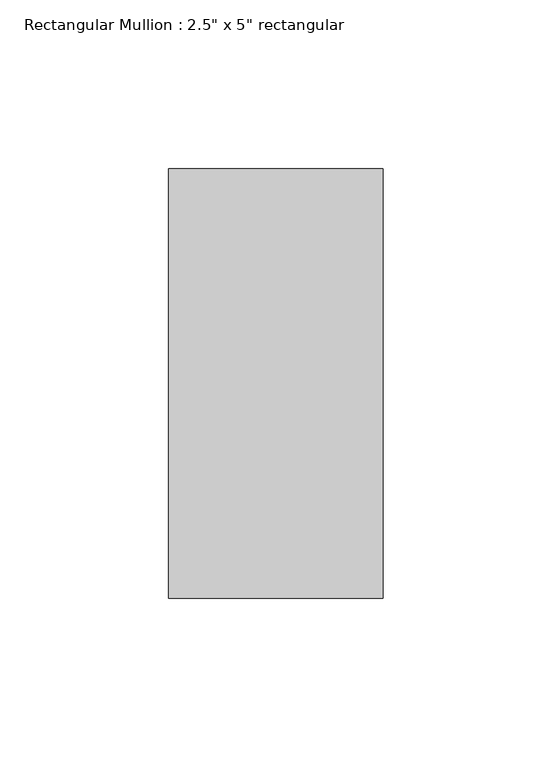
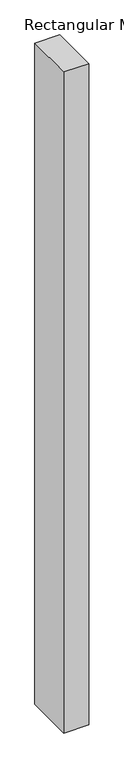
"""IFC4 building model written with IfcOpenShell, lengths in millimetres: member geometry."""

from ifc_helpers import new_model, si_unit, frame, origin, place, context, project, spatial, polyline, outline, extrude, source, transform, mapped, element, save


def member_c04b3d4e(model_context):
    return source(origin(), model_context, "Body", "SweptSolid", [
        extrude(outline(polyline([(0.0, 63.5), (0.0, -63.5), (-63.5, -63.5), (-63.5, 63.5), (0.0, 63.5)])), frame((0.0, 0.0, -1779.2221241), z_axis=(0.0, 0.0, 1.0), x_axis=(1.0, 0.0, 0.0)), (0.0, 0.0, 1.0), 1779.2221241),
    ])


if __name__ == "__main__":
    model = new_model("IFC4")
    model_context = context("Model", 3, world=origin())
    ifc_project = project(units=[si_unit("LENGTHUNIT", "METRE", prefix="MILLI")], contexts=[model_context])
    site = spatial("IfcSite", under=ifc_project)
    building = spatial("IfcBuilding", under=site)
    placement = place(None, origin())
    member_shape = member_c04b3d4e(model_context)
    element("IfcMember", 1, ObjectType="Rectangular Mullion : 2.5\" x 5\" rectangular", at=placement, inside=building, context=model_context, shape_type="MappedRepresentation", body=[
        mapped(member_shape, transform((0.0, 0.0, 0.0), x_axis=(1.0, 0.0, 0.0), y_axis=(0.0, 1.0, 0.0), z_axis=(0.0, 0.0, 1.0))),
    ])
    save(model, "model.ifc")

# Revit data of these elements
# Type "Rectangular Mullion : 2.5\" x 5\" rectangular"
#   built-in parameter 1007304 = 0.416667 (stored number, unit not read)
#   built-in parameter 1007301 = 0.104167 (stored number, unit not read)
#   built-in parameter 1007300 = 0.104167 (stored number, unit not read)
# Element 1 (IfcMember, "Rectangular Mullion : 2.5\" x 5\" rectangular")
#   Materials on its faces: "Aluminum"
# Materials
#   "Aluminum": class "Metal", colour RGB 247 247 247, transparency 0, Description = "Aluminum 6061", Cost = 0
